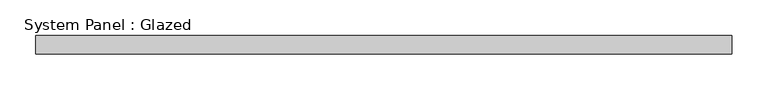
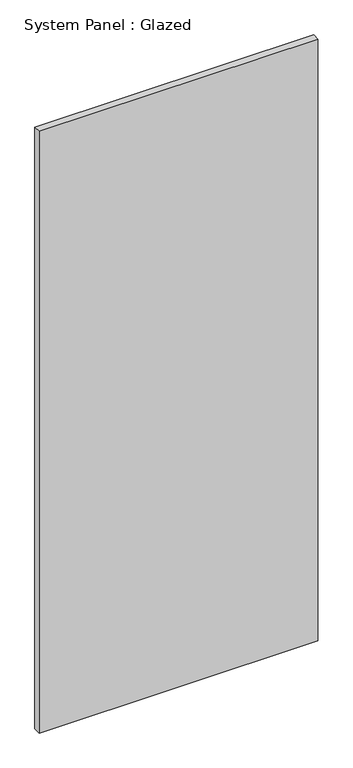
"""IFC4 building model written with IfcOpenShell, lengths in millimetres: plate geometry, System Panel : Glazed."""

from ifc_helpers import new_model, si_unit, origin, origin_with_axes, place, context, project, spatial, polyline, outline, extrude, source, transform, mapped, element, save


def system_panel_glazed_afec1f6d(model_context):
    return source(origin(), model_context, "Body", "SweptSolid", [
        extrude(outline(polyline([(485.775, 19.05), (-485.775, 19.05), (-485.775, 44.45), (485.775, 44.45), (485.775, 19.05)])), origin_with_axes(), (0.0, 0.0, 1.0), 2216.9308081),
    ])


if __name__ == "__main__":
    model = new_model("IFC4")
    model_context = context("Model", 3, world=origin())
    ifc_project = project(units=[si_unit("LENGTHUNIT", "METRE", prefix="MILLI")], contexts=[model_context])
    site = spatial("IfcSite", under=ifc_project)
    building = spatial("IfcBuilding", under=site)
    placement = place(None, origin())
    system_panel_glazed_shape = system_panel_glazed_afec1f6d(model_context)
    element("IfcPlate", 1, ObjectType="System Panel : Glazed", at=placement, inside=building, context=model_context, shape_type="MappedRepresentation", body=[
        mapped(system_panel_glazed_shape, transform((0.0, 0.0, 0.0), x_axis=(1.0, 0.0, 0.0), y_axis=(0.0, 1.0, 0.0), z_axis=(0.0, 0.0, 1.0))),
    ])
    save(model, "model.ifc")

# Revit data of these elements
# Type "System Panel : Glazed"
#   Construction Type Id = "GSP4R"
#   Analytic Construction = "1/8 in Pilkington single glazing"
#   Visual Light Transmittance = 0.9
#   Solar Heat Gain Coefficient = 0.86
#   Heat Transfer Coefficient (U) = 1.18115 BTU/(h·ft²·°F)
#   Define Thermal Properties by = 1
# Element 1 (IfcPlate, "System Panel : Glazed")
#   Materials on its faces: "Glass"
# Materials
#   "Glass": class "Glass", colour RGB 0 128 192, transparency 0.75, Description = "Soda Lime Glass", Cost = 0
